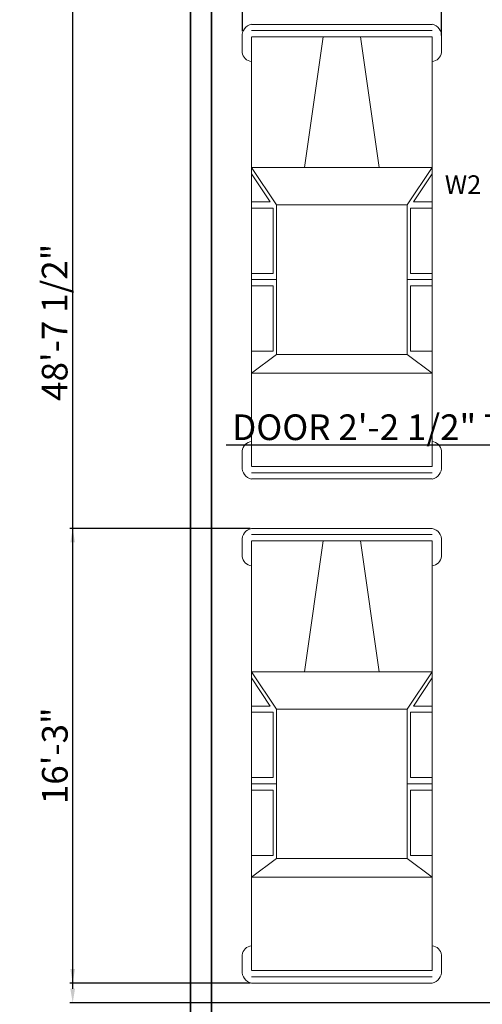
# Model space of a CAD drawing. Units: inches. Extents: x 2069 to 3028, y 691 to 1726.
# Tile 2 of 10: x 2069 to 2267, y 903 to 1325. Entities that reach past the tile are written whole.
import ezdxf

# ---------------------------------------------------------------- set-up
doc = ezdxf.new("R2010")
doc.units = ezdxf.units.IN
doc.layers.add('A-ANNO-DIMS', color=2, linetype='Continuous', lineweight=18)
doc.layers.add('L-SITE-WALL', color=7, linetype='Continuous', lineweight=35)
doc.layers.add('A-ANNO-TEXT', color=11, linetype='Continuous', lineweight=18, true_color=0xf27172)
doc.layers.add('C-SITE-VEHI', color=2, linetype='Continuous', lineweight=13, true_color=0xf1eb1f)
doc.styles.get("Standard").update_dxf_attribs({"font": 'arial.ttf'})
doc.dimstyles.new('ISO-25', dxfattribs={"dimtxt": 11, "dimasz": 6, "dimexe": 1.25, "dimexo": 0.625, "dimtad": 1, "dimlunit": 3, "dimtxsty": 'Standard', "dimcen": 2.5, "dimclrd": 3, "dimclre": 5, "dimclrt": 6, "dimadec": 0, "dimazin": 0, "dimtfac": 1, "dimtmove": 0, "dimatfit": 3, "dimfxl": 1, "dimarcsym": 0})

# ---------------------------------------------------------------- blocks, each defined once
blk = doc.blocks.new('*U13')
for p, q in [((138, 1075), (308, 1075)), ((4818, 1075), (4649, 1075)), ((3, -10), (3, 974)), ((70, -10), (70, 973)), ((138, 973), (410, 973)), ((138, -10), (138, 971)), ((410, 973), (4581, 973)), ((1563, -10), (1563, 973)), ((1563, 973), (1969, 702)), ((1630, 973), (1936, 769)), ((1936, 769), (1936, 973)), ((2003, 973), (2003, 736)), ((2716, 736), (2716, 973)), ((2783, 702), (2783, 973)), ((2851, 973), (2851, 736)), ((3563, 736), (3563, 973)), ((3597, 702), (3801, 973)), ((3801, -10), (3801, 973)), ((4818, 973), (4547, 973)), ((4818, -10), (4818, 971)), ((4886, -10), (4886, 973)), ((4954, -10), (4954, 974)), ((1969, 702), (3597, 702)), ((1969, -10), (1969, 702)), ((2003, 736), (2716, 736)), ((2851, 736), (3563, 736)), ((3597, -10), (3597, 702)), ((138, 193), (1563, 396)), ((3, -11), (3, -995)), ((70, -10), (70, -994)), ((138, -11), (138, -992)), ((1563, -10), (1563, -994)), ((1969, -10), (1969, -723)), ((3597, -10), (3597, -723)), ((3801, -10), (3801, -994)), ((4818, -11), (4818, -992)), ((4886, -10), (4886, -994)), ((4954, -11), (4954, -995)), ((138, -214), (1563, -417)), ((1563, -994), (1969, -723)), ((1969, -723), (3597, -723)), ((2783, -723), (2783, -994)), ((3597, -723), (3801, -994)), ((1630, -994), (1936, -790)), ((1936, -790), (1936, -994)), ((2003, -994), (2003, -757)), ((2003, -757), (2716, -757)), ((2716, -757), (2716, -994)), ((2851, -757), (3563, -757)), ((2851, -994), (2851, -757)), ((3563, -757), (3563, -994)), ((138, -994), (410, -994)), ((410, -994), (4581, -994)), ((4818, -994), (4547, -994)), ((138, -1096), (308, -1096)), ((4818, -1096), (4649, -1096))]:
    blk.add_line(p, q)
for centre, radius, start, end in [((128, 946), 129, 85.6455, 168.0943), ((291, 956), 120, 8.1301, 81.87), ((4665, 956), 120, 98.13, 171.8699), ((4828, 946), 129, 11.9057, 94.3545), ((128, -967), 129, 191.9057, 274.3545), ((291, -977), 120, 278.13, 351.8699), ((4665, -977), 120, 188.1301, 261.87), ((4828, -967), 129, 265.6455, 348.0943)]:
    blk.add_arc(centre, radius, start, end)
blk = doc.blocks.new('*D64')
at = {"layer": 'A-ANNO-DIMS', "color": 5, "lineweight": -2, "transparency": 16777216}
for p, q in [((2306.95, 1146.26), (2306.95, 1141.66)), ((2333.49, 1146.26), (2333.49, 1141.66))]:
    blk.add_line(p, q, dxfattribs=at)
at = {"layer": 'A-ANNO-DIMS', "color": 3, "lineweight": -2, "transparency": 16777216}
for p, q in [((2306.95, 1142.91), (2157.2, 1142.91)), ((2327.49, 1142.91), (2312.95, 1142.91))]:
    blk.add_line(p, q, dxfattribs=at)
at = {"layer": 'A-ANNO-DIMS', "color": 3, "transparency": 16777216}
for points in [[(2312.95, 1143.91), (2312.95, 1141.91), (2306.95, 1142.91)], [(2327.49, 1143.91), (2327.49, 1141.91), (2333.49, 1142.91)]]:
    blk.add_solid(points, dxfattribs=at)
at = {"layer": 'Defpoints', "color": 0, "transparency": 16777216}
for p in [(2306.95, 1146.89), (2333.49, 1146.89), (2306.95, 1142.91)]:
    blk.add_point(p, dxfattribs=at)
at = {"layer": 'A-ANNO-DIMS', "color": 6, "transparency": 16777216, "insert": (2229.07, 1149.22), "char_height": 11, "attachment_point": 5}
blk.add_mtext('DOOR 2\'-2 1/2" TYP.', dxfattribs=at)
blk = doc.blocks.new('*D87')
at = {"layer": 'A-ANNO-DIMS', "color": 5, "lineweight": -2, "transparency": 16777216}
for p, q in [((2297.33, 1487.39), (2090.2, 1487.39)), ((2297.33, 903.89), (2090.2, 903.89))]:
    blk.add_line(p, q, dxfattribs=at)
at = {"layer": 'A-ANNO-DIMS', "color": 3, "lineweight": -2, "transparency": 16777216}
blk.add_line((2091.45, 909.89), (2091.45, 1481.39), dxfattribs=at)
at = {"layer": 'A-ANNO-DIMS', "color": 3, "transparency": 16777216}
for points in [[(2090.45, 1481.39), (2092.45, 1481.39), (2091.45, 1487.39)], [(2090.45, 909.89), (2092.45, 909.89), (2091.45, 903.89)]]:
    blk.add_solid(points, dxfattribs=at)
at = {"layer": 'Defpoints', "color": 0, "transparency": 16777216}
for p in [(2091.45, 1487.39), (2297.95, 1487.39), (2297.95, 903.89)]:
    blk.add_point(p, dxfattribs=at)
at = {"layer": 'A-ANNO-DIMS', "color": 6, "transparency": 16777216, "insert": (2085.14, 1195.64), "char_height": 11, "attachment_point": 5, "rotation": 90}
blk.add_mtext('48\'-7 1/2"', dxfattribs=at)
blk = doc.blocks.new('*D93')
at = {"layer": 'A-ANNO-DIMS', "color": 5, "lineweight": -2, "transparency": 16777216}
for p, q in [((2167.44, 1107.24), (2090.2, 1107.24)), ((2167.44, 912.32), (2090.2, 912.32))]:
    blk.add_line(p, q, dxfattribs=at)
at = {"layer": 'A-ANNO-DIMS', "color": 3, "lineweight": -2, "transparency": 16777216}
blk.add_line((2091.45, 918.32), (2091.45, 1101.24), dxfattribs=at)
at = {"layer": 'A-ANNO-DIMS', "color": 3, "transparency": 16777216}
for points in [[(2090.45, 1101.24), (2092.45, 1101.24), (2091.45, 1107.24)], [(2090.45, 918.32), (2092.45, 918.32), (2091.45, 912.32)]]:
    blk.add_solid(points, dxfattribs=at)
at = {"layer": 'Defpoints', "color": 0, "transparency": 16777216}
for p in [(2091.45, 1107.24), (2168.07, 1107.24), (2168.07, 912.32)]:
    blk.add_point(p, dxfattribs=at)
at = {"layer": 'A-ANNO-DIMS', "color": 6, "transparency": 16777216, "insert": (2085.21, 1009.78), "char_height": 11, "attachment_point": 5, "rotation": 90}
blk.add_mtext('16\'-3"', dxfattribs=at)
blk = doc.blocks.new('*D94')
at = {"layer": 'A-ANNO-DIMS', "color": 5, "lineweight": -2, "transparency": 16777216}
for p, q in [((2164.26, 1320.51), (2164.26, 1704.14)), ((2249.51, 1318.68), (2249.51, 1704.14))]:
    blk.add_line(p, q, dxfattribs=at)
at = {"layer": 'A-ANNO-DIMS', "color": 3, "lineweight": -2, "transparency": 16777216}
blk.add_line((2170.26, 1702.89), (2243.51, 1702.89), dxfattribs=at)
at = {"layer": 'A-ANNO-DIMS', "color": 3, "transparency": 16777216}
for points in [[(2170.26, 1703.89), (2170.26, 1701.89), (2164.26, 1702.89)], [(2243.51, 1703.89), (2243.51, 1701.89), (2249.51, 1702.89)]]:
    blk.add_solid(points, dxfattribs=at)
at = {"layer": 'Defpoints', "color": 0, "transparency": 16777216}
for p in [(2249.51, 1702.89), (2164.26, 1319.89), (2249.51, 1318.06)]:
    blk.add_point(p, dxfattribs=at)
at = {"layer": 'A-ANNO-DIMS', "color": 6, "transparency": 16777216, "insert": (2206.88, 1709.2), "char_height": 11, "attachment_point": 5}
blk.add_mtext('7\'-1 1/2"', dxfattribs=at)

msp = doc.modelspace()

# ---------------------------------------------------------------- linework, layer by layer
at = {"layer": 'L-SITE-WALL'}
for p, q in [((2141.951, 1652.387), (2141.951, 737.387)), ((2150.951, 1535.387), (2150.951, 746.387))]:
    msp.add_line(p, q, dxfattribs=at)

# ---------------------------------------------------------------- block references
at = {"layer": 'C-SITE-VEHI', "xscale": 0.0393700787401575, "yscale": 0.0393700787401575, "zscale": 0.0393700787401575, "rotation": 270}
for p in [(2207.199, 1323.501), (2207.199, 1107.346)]:
    msp.add_blockref('*U13', p, dxfattribs=at)

# ---------------------------------------------------------------- texts
at = {"layer": 'A-ANNO-TEXT', "insert": (2250.905, 1258.661), "char_height": 8, "attachment_point": 1}
msp.add_mtext_dynamic_manual_height_columns('{\\fArial|b1|i0|c0|p34;W2}', width=34.05605, gutter_width=12.5, heights=[0], dxfattribs=at)

# ---------------------------------------------------------------- dimensions: what is measured, and where the dimension line sits
at = {"layer": 'A-ANNO-DIMS'}
dim = msp.add_linear_dim(base=(2249.51, 1702.887), p1=(2164.257, 1319.887), p2=(2249.51, 1318.058), dimstyle='ISO-25', override={"dimdec": 1, "dimlfac": 1, "dimrnd": 0, "dimzin": 1, "dimdsep": 46, "dimlunit": 4, "dimfrac": 2}, dxfattribs=at)
dim.commit()
dim.dimension.update_dxf_attribs({"geometry": '*D94', "text_midpoint": (2206.884, 1709.199)})
for base, p1, p2, picture, middle in [((2091.451, 1487.387), (2297.951, 903.887), (2297.951, 1487.387), '*D87', (2085.139, 1195.637)), ((2091.451, 1107.244), (2168.068, 912.317), (2168.068, 1107.244), '*D93', (2085.206, 1009.78))]:
    dim = msp.add_linear_dim(base=base, p1=p1, p2=p2, angle=90, dimstyle='ISO-25', override={"dimdec": 1, "dimlfac": 1, "dimrnd": 0, "dimzin": 1, "dimdsep": 46, "dimlunit": 4, "dimfrac": 2}, dxfattribs=at)
    dim.commit()
    dim.dimension.update_dxf_attribs({"geometry": picture, "text_midpoint": middle})
dim = msp.add_linear_dim(base=(2306.951, 1142.906), p1=(2333.487, 1146.887), p2=(2306.951, 1146.887), angle=180, text='DOOR <> TYP.', dimstyle='ISO-25', override={"dimdec": 1, "dimlfac": 1, "dimrnd": 0, "dimzin": 1, "dimdsep": 46, "dimlunit": 4, "dimfrac": 2}, dxfattribs=at)
dim.commit()
dim.dimension.update_dxf_attribs({"geometry": '*D64', "text_midpoint": (2229.074, 1149.222)})

doc.saveas('drawing.dxf')
